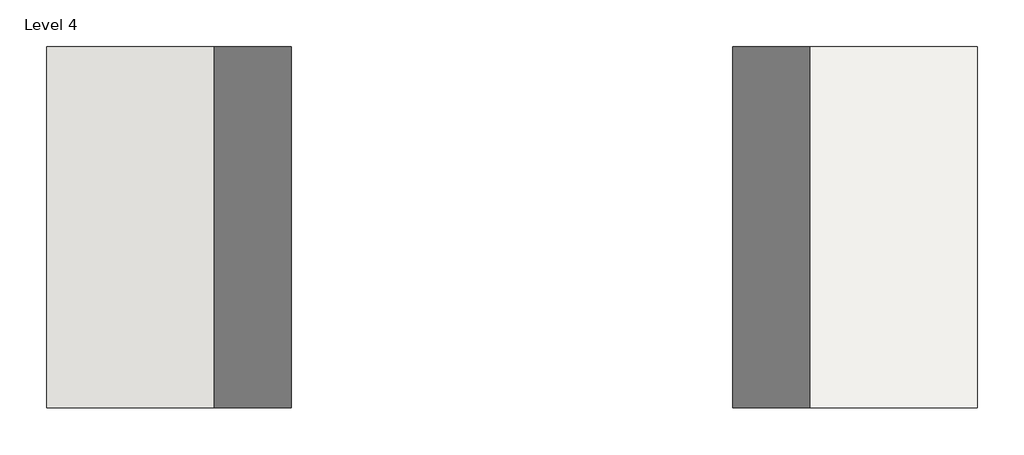
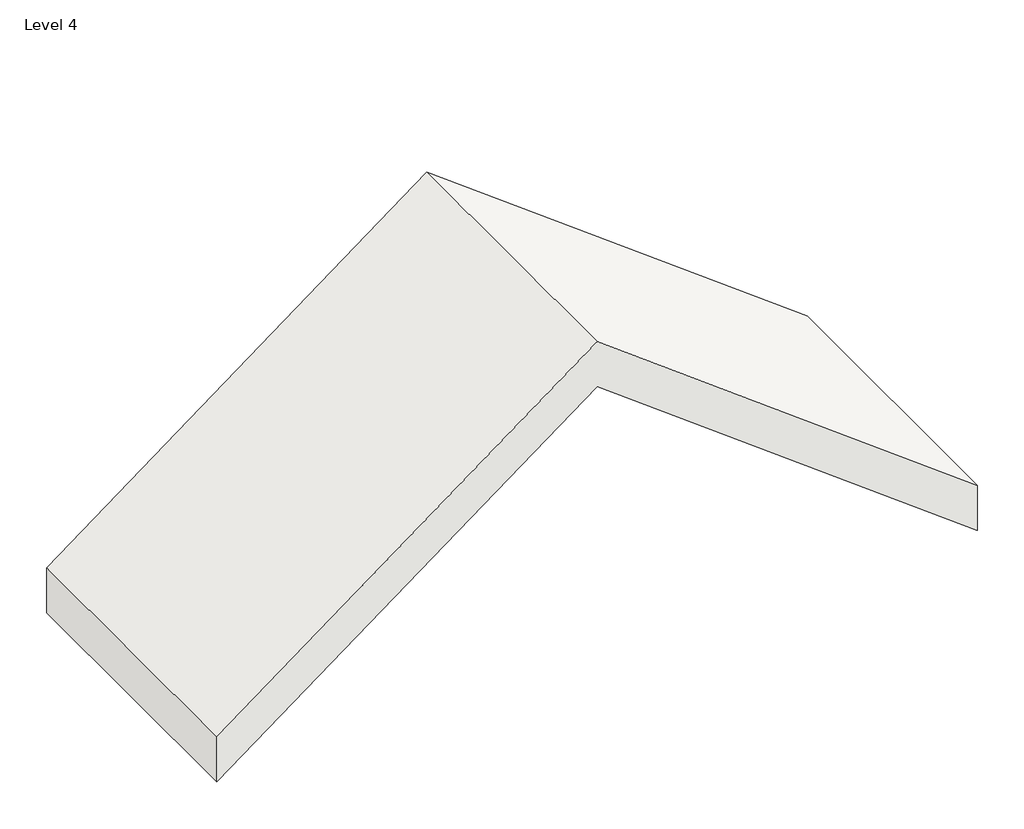
# One storey: 1 roof.
"""IFC4 building model written with IfcOpenShell, lengths in millimetres."""

from ifc_helpers import new_model, si_unit, frame, origin, place, context, project, spatial, polyline, outline, extrude, element, save

model = new_model("IFC4")

# Units and contexts
model_context = context("Model", 3, world=origin())
ifc_project = project(units=[si_unit("LENGTHUNIT", "METRE", prefix="MILLI")], contexts=[model_context])

# Site, building, storey
site = spatial("IfcSite", under=ifc_project)
building = spatial("IfcBuilding", under=site)
storey = spatial("IfcBuildingStorey", under=building, Name="Level 4", Elevation=9144.0)

# Roof
placement = place(None, origin())
element("IfcRoof", 1, ObjectType="Generic - 12\"", at=placement, inside=storey, context=model_context, shape_type="SweptSolid", body=[
    extrude(outline(polyline([(9525.0, -4720.2032698), (11806.7253039, -7762.503675), (9525.0, -10804.8040802), (9144.0, -10804.8040802), (11425.7253039, -7762.503675), (9144.0, -4720.2032698), (9525.0, -4720.2032698)])), frame((0.0, -13088.6518738, 0.0), z_axis=(0.0, 1.0, 0.0), x_axis=(0.0, 0.0, 1.0)), (0.0, 0.0, 1.0), 2362.2),
])

save(model, "model.ifc")

# Revit data of these elements
# Type "Generic - 12\""
#   Assembly Code = "B1020"
#   Layers, outside or top first: 1' - 0" no material (function 1)
# Element 1 (IfcRoof, "Generic - 12\"")
#   built-in parameter 1001705 = 38.736 (stored number, unit not read)
#   built-in parameter 1001710 = 33615
#   Phase Created = New Construction
#   Materials on its faces: "Default Roof"
# Materials
#   "Default Roof": colour RGB 88 101 114, transparency 0, Cost = 0
